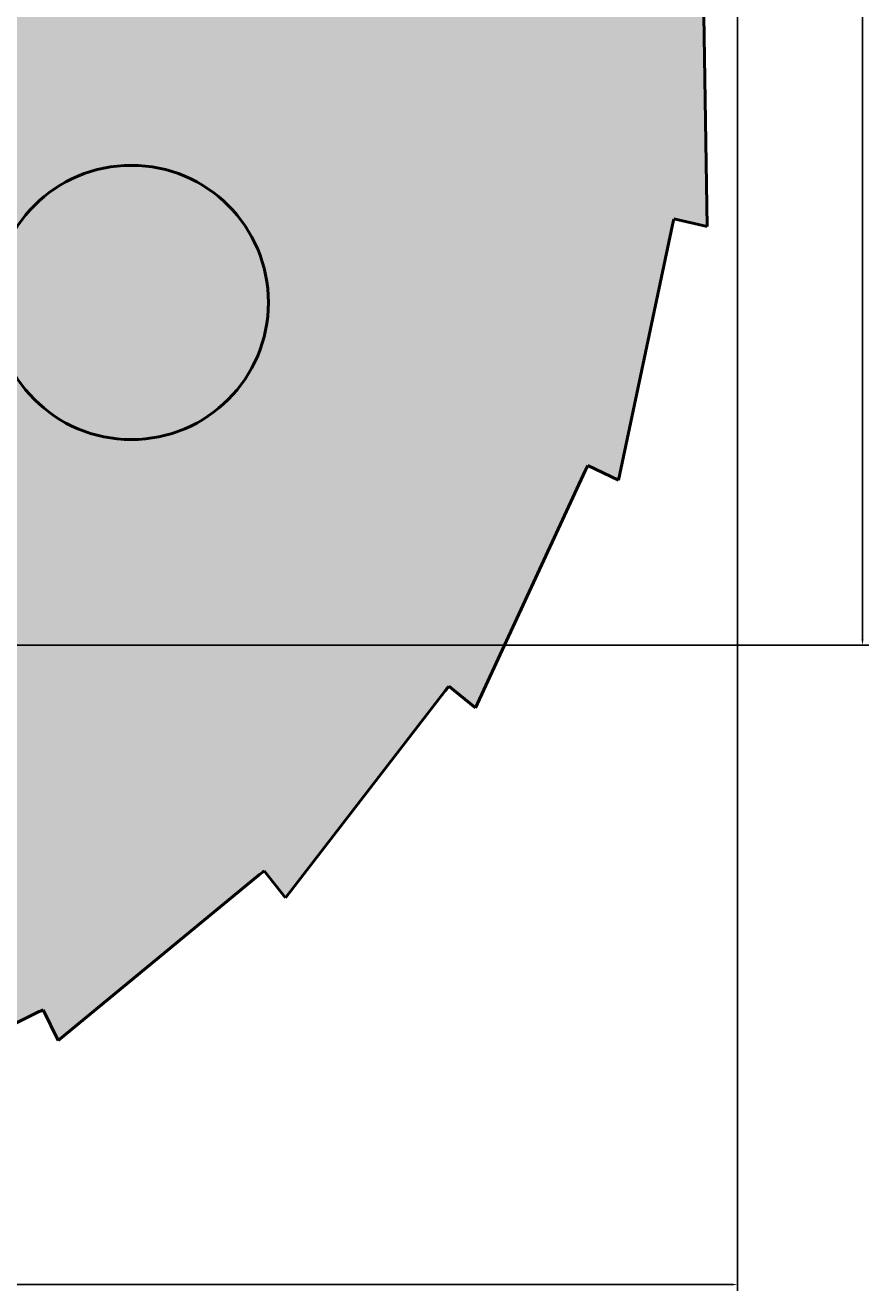
# Model space of a CAD drawing. Units: millimetres. Extents: x 2943.6 to 3032.7, y 1562 to 1639.7.
# Tile 7 of 9: x 2996.7 to 3021.3, y 1562 to 1598.9. Entities that reach past the tile are written whole.
import ezdxf

# ---------------------------------------------------------------- set-up
doc = ezdxf.new("R2010")
doc.units = ezdxf.units.MM
doc.layers.add('M-DIMS', color=2, linetype='Continuous', lineweight=18)
doc.layers.add('M-OUTL', color=7, linetype='Continuous', lineweight=50)
doc.layers.add('M-HATC', color=7, linetype='Continuous', lineweight=18, true_color=0xffffff)
doc.styles.get("Standard").update_dxf_attribs({"font": 'arial.ttf'})
doc.dimstyles.get("Standard").update_dxf_attribs({"dimtxt": 0.18, "dimasz": 0.18, "dimexe": 0.18, "dimexo": 0.0625, "dimgap": 0.09, "dimtad": 0, "dimtih": 1, "dimtoh": 1, "dimdec": 4, "dimzin": 0, "dimdsep": 46, "dimtxsty": 'Standard', "dimcen": 0.09, "dimadec": 0, "dimazin": 0, "dimtfac": 1, "dimtdec": 4, "dimtofl": 0, "dimtmove": 0, "dimatfit": 3, "dimfxl": 1, "dimtolj": 1, "dimtzin": 0, "dimarcsym": 0})

# ---------------------------------------------------------------- blocks, each defined once
blk = doc.blocks.new('*U1')
blk.add_circle((0, 0), 4)
blk = doc.blocks.new('*U2')
at = {"layer": 'M-OUTL', "color": 0, "linetype": 'ByBlock', "lineweight": -2, "transparency": 16777216, "rotation": 240}
blk.add_blockref('*U1', (2999.79, 1590.848), dxfattribs=at)
blk = doc.blocks.new('*D3')
at = {"layer": 'Defpoints', "color": 0, "transparency": 16777216}
for p in [(2947.469, 1600.848), (3017.469, 1600.848), (3017.469, 1562.198)]:
    blk.add_point(p, dxfattribs=at)
at = {"layer": 'M-DIMS', "color": 0, "lineweight": -2, "transparency": 16777216}
for p, q in [((2947.469, 1600.786), (2947.469, 1562.018)), ((3017.469, 1600.786), (3017.469, 1562.018)), ((2947.649, 1562.198), (2982.251, 1562.198)), ((3017.289, 1562.198), (2982.687, 1562.198))]:
    blk.add_line(p, q, dxfattribs=at)
at = {"layer": 'M-DIMS', "color": 0, "transparency": 16777216}
for points in [[(2947.649, 1562.228), (2947.649, 1562.168), (2947.469, 1562.198)], [(3017.289, 1562.228), (3017.289, 1562.168), (3017.469, 1562.198)]]:
    blk.add_solid(points, dxfattribs=at)
at = {"layer": 'M-DIMS', "color": 0, "transparency": 16777216, "insert": (2982.469, 1562.198), "char_height": 0.18, "attachment_point": 5}
blk.add_mtext('\\A1;70', dxfattribs=at)
blk = doc.blocks.new('*D5')
at = {"layer": 'Defpoints', "color": 0, "transparency": 16777216}
for p in [(2986.469, 1620.848), (3021.119, 1620.848), (2986.469, 1580.848)]:
    blk.add_point(p, dxfattribs=at)
at = {"layer": 'M-DIMS', "color": 0, "lineweight": -2, "transparency": 16777216}
for p, q in [((2986.532, 1620.848), (3021.299, 1620.848)), ((3021.119, 1620.668), (3021.119, 1601.03)), ((3021.119, 1581.028), (3021.119, 1600.666)), ((2986.532, 1580.848), (3021.299, 1580.848))]:
    blk.add_line(p, q, dxfattribs=at)
at = {"layer": 'M-DIMS', "color": 0, "transparency": 16777216}
for points in [[(3021.089, 1620.668), (3021.149, 1620.668), (3021.119, 1620.848)], [(3021.089, 1581.028), (3021.149, 1581.028), (3021.119, 1580.848)]]:
    blk.add_solid(points, dxfattribs=at)
at = {"layer": 'M-DIMS', "color": 0, "transparency": 16777216, "insert": (3021.119, 1600.848), "char_height": 0.18, "attachment_point": 5}
blk.add_mtext('\\A1;40', dxfattribs=at)

msp = doc.modelspace()

# ---------------------------------------------------------------- hatches: boundary and pattern name
at = {"layer": 'M-HATC'}
h = msp.add_hatch(color=256, dxfattribs=at)
h.set_gradient(color1=(0, 0, 255), color2=(255, 255, 0), tint=1, name='INVCURVED')
h.paths.add_polyline_path([(2949.361, 1608.583, 0.001279), (2949.322, 1608.414), (2948.347, 1608.637), (2948.473, 1600.848), (2947.469, 1600.848), (2949.283, 1593.452, 0.001279), (2949.322, 1593.283), (2948.347, 1593.06), (2951.761, 1586.253, 0.001279), (2951.836, 1586.096), (2950.935, 1585.662), (2955.779, 1579.786, 0.001279), (2955.887, 1579.65), (2955.105, 1579.026), (2961.135, 1574.375, 0.001279), (2961.271, 1574.266), (2960.647, 1573.484), (2967.561, 1570.291, 0.001279), (2967.717, 1570.215), (2967.283, 1569.314), (2974.734, 1567.74, 0.001279), (2974.904, 1567.701), (2974.681, 1566.726), (2982.295, 1566.849, 0.001279), (2982.469, 1566.848), (2982.469, 1565.848), (2989.865, 1567.662, 0.001279), (2990.035, 1567.701), (2990.258, 1566.726), (2997.064, 1570.14, 0.001279), (2997.221, 1570.215), (2997.655, 1569.314), (3003.532, 1574.158, 0.001279), (3003.668, 1574.266), (3004.291, 1573.484), (3008.943, 1579.514, 0.001279), (3009.052, 1579.65), (3009.833, 1579.026), (3013.026, 1585.94, 0.001279), (3013.102, 1586.096), (3014.003, 1585.662), (3015.578, 1593.113, 0.001279), (3015.617, 1593.283), (3016.592, 1593.06), (3016.469, 1600.674, 0.001279), (3016.469, 1600.848), (3017.469, 1600.848), (3015.655, 1608.244, 0.001279), (3015.617, 1608.414), (3016.592, 1608.637), (3013.177, 1615.443, 0.001279), (3013.102, 1615.6), (3014.003, 1616.034), (3009.16, 1621.911, 0.001279), (3009.052, 1622.047), (3009.833, 1622.67), (3003.804, 1627.322, 0.001279), (3003.668, 1627.431), (3004.291, 1628.212), (2997.378, 1631.405, 0.001279), (2997.221, 1631.481), (2997.655, 1632.382), (2990.204, 1633.957, 0.001279), (2990.035, 1633.996), (2990.258, 1634.971), (2982.469, 1634.845), (2982.469, 1635.848), (2975.073, 1634.034, 0.001279), (2974.904, 1633.996), (2974.681, 1634.971), (2967.874, 1631.556, 0.001279), (2967.717, 1631.481), (2967.283, 1632.382), (2961.407, 1627.539, 0.001279), (2961.271, 1627.431), (2960.647, 1628.212), (2955.996, 1622.183, 0.001279), (2955.887, 1622.047), (2955.105, 1622.67), (2951.912, 1615.757, 0.001279), (2951.836, 1615.6), (2950.935, 1616.034)])
h.paths.add_polyline_path([(2969.149, 1610.848, -1), (2961.149, 1610.848, -1)], flags=16)
h.paths.add_polyline_path([(2969.149, 1590.848, -1), (2961.149, 1590.848, -1)], flags=16)
h.paths.add_polyline_path([(2992.469, 1600.848, -1), (2972.469, 1600.848, -1)], flags=16)
h.paths.add_polyline_path([(2978.469, 1620.848, -1), (2986.469, 1620.848, -1)], flags=16)
h.paths.add_polyline_path([(2981.469, 1605.236), (2981.469, 1606.848), (2983.469, 1606.848), (2983.469, 1605.236, -8.887482)], flags=0)
h.paths.add_polyline_path([(2986.469, 1580.848, -1), (2978.469, 1580.848, -1)], flags=16)
h.paths.add_polyline_path([(3003.79, 1610.848, -1), (2995.79, 1610.848, -1)], flags=16)
h.paths.add_polyline_path([(3003.79, 1590.848, -1), (2995.79, 1590.848, -1)], flags=16)
h = msp.add_hatch(color=256, dxfattribs=at)
h.paths.add_polyline_path([(2978.469, 1620.848, 1), (2986.469, 1620.848, 1)])
h.paths.add_polyline_path([(2995.79, 1610.848, 1), (3003.79, 1610.848, 1)])
h.paths.add_polyline_path([(3003.79, 1590.848, 1), (2995.79, 1590.848, 1)])
h.paths.add_polyline_path([(2986.469, 1580.848, 1), (2978.469, 1580.848, 1)])
h.paths.add_polyline_path([(2969.149, 1590.848, 1), (2961.149, 1590.848, 1)])
h.paths.add_polyline_path([(2961.149, 1610.848, 1), (2969.149, 1610.848, 1)])

# ---------------------------------------------------------------- linework, layer by layer
at = {"layer": 'M-OUTL'}
for p, q in [((3016.469, 1600.674), (3016.592, 1593.06)), ((3015.617, 1593.283), (3016.592, 1593.06)), ((3015.578, 1593.113), (3014.003, 1585.662)), ((3013.026, 1585.94), (3009.833, 1579.026)), ((3013.102, 1586.096), (3014.003, 1585.662)), ((3009.052, 1579.65), (3009.833, 1579.026)), ((3008.943, 1579.514), (3004.291, 1573.484)), ((3003.532, 1574.158), (2997.655, 1569.314)), ((3003.668, 1574.266), (3004.291, 1573.484)), ((2997.064, 1570.14), (2990.258, 1566.726)), ((2997.221, 1570.215), (2997.655, 1569.314))]:
    msp.add_line(p, q, dxfattribs=at)
for start, end in [(346.8498, 347.1429), (333.9926, 334.2857), (321.1355, 321.4286), (308.2783, 308.5714), (295.4212, 295.7143)]:
    msp.add_arc((2982.469, 1600.848), 34, start, end, dxfattribs=at)

# ---------------------------------------------------------------- block references
msp.add_blockref('*U2', (0, 0), dxfattribs=at)

# ---------------------------------------------------------------- dimensions: what is measured, and where the dimension line sits
at = {"layer": 'M-DIMS'}
dim = msp.add_linear_dim(base=(3021.119, 1620.848), p1=(2986.469, 1580.848), p2=(2986.469, 1620.848), angle=90, dimstyle='Standard', override={"dimdec": 0, "dimlfac": 1, "dimrnd": 0, "dimzin": 0, "dimdsep": 46, "dimlunit": 2}, dxfattribs=at)
dim.commit()
dim.dimension.update_dxf_attribs({"geometry": '*D5', "text_midpoint": (3021.119, 1600.848)})
dim = msp.add_linear_dim(base=(3017.469, 1562.198), p1=(2947.469, 1600.848), p2=(3017.469, 1600.848), dimstyle='Standard', override={"dimdec": 0, "dimlfac": 1, "dimrnd": 0, "dimzin": 0, "dimdsep": 46, "dimlunit": 2}, dxfattribs=at)
dim.commit()
dim.dimension.update_dxf_attribs({"geometry": '*D3', "text_midpoint": (2982.469, 1562.198)})

doc.saveas('drawing.dxf')
